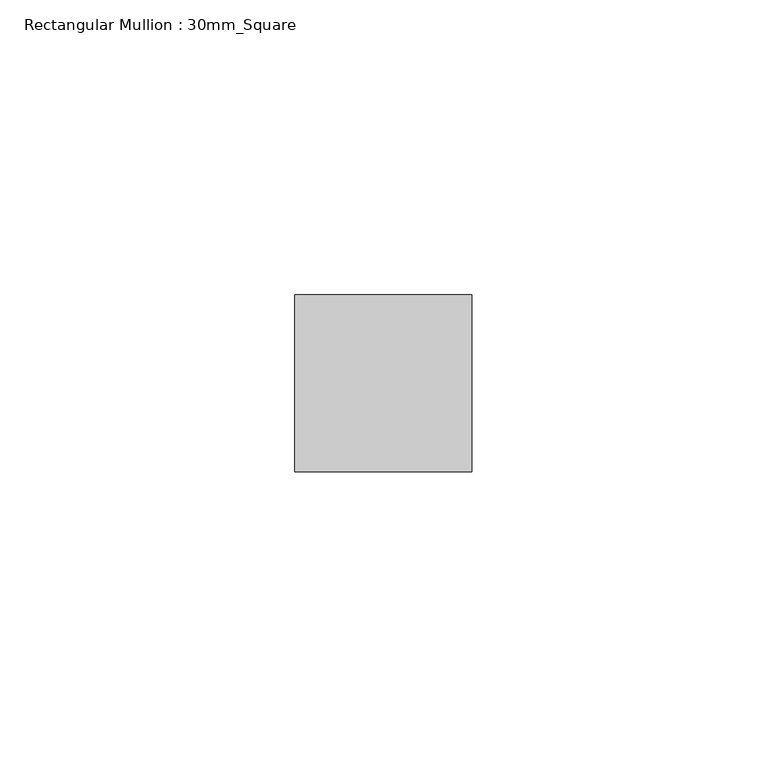
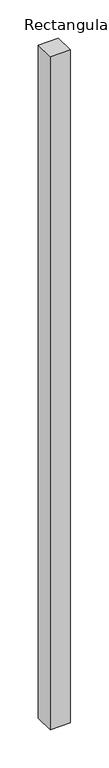
"""IFC4 building model written with IfcOpenShell, lengths in millimetres: member geometry, Rectangular Mullion : 30mm_Square."""

from ifc_helpers import new_model, si_unit, frame, origin, place, context, project, spatial, polyline, outline, extrude, source, transform, mapped, element, save


def rectangular_mullion_30mm_square_457ab78e(model_context):
    return source(origin(), model_context, "Body", "SweptSolid", [
        extrude(outline(polyline([(15.0, 15.0), (15.0, -15.0), (-15.0, -15.0), (-15.0, 15.0), (15.0, 15.0)])), frame((0.0, 0.0, -1067.1518548), z_axis=(0.0, 0.0, 1.0), x_axis=(1.0, 0.0, 0.0)), (0.0, 0.0, 1.0), 1067.1518548),
    ])


if __name__ == "__main__":
    model = new_model("IFC4")
    model_context = context("Model", 3, world=origin())
    ifc_project = project(units=[si_unit("LENGTHUNIT", "METRE", prefix="MILLI")], contexts=[model_context])
    site = spatial("IfcSite", under=ifc_project)
    building = spatial("IfcBuilding", under=site)
    placement = place(None, origin())
    rectangular_mullion_30mm_square_shape = rectangular_mullion_30mm_square_457ab78e(model_context)
    element("IfcMember", 1, ObjectType="Rectangular Mullion : 30mm_Square", at=placement, inside=building, context=model_context, shape_type="MappedRepresentation", body=[
        mapped(rectangular_mullion_30mm_square_shape, transform((0.0, 0.0, 0.0), x_axis=(1.0, 0.0, 0.0), y_axis=(0.0, 1.0, 0.0), z_axis=(0.0, 0.0, 1.0))),
    ])
    save(model, "model.ifc")

# Revit data of these elements
# Type "Rectangular Mullion : 30mm_Square"
#   Keynote = "H11"
#   built-in parameter 1007304 = 0.0984252 (stored number, unit not read)
#   built-in parameter 1007301 = 0.0492126 (stored number, unit not read)
#   built-in parameter 1007300 = 0.0492126 (stored number, unit not read)
# Element 1 (IfcMember, "Rectangular Mullion : 30mm_Square")
#   Materials on its faces: "Aluminium"
# Materials
#   "Aluminium": class "Metal", colour RGB 247 247 247, transparency 0, Description = "Aluminium 6061", Cost = 0
